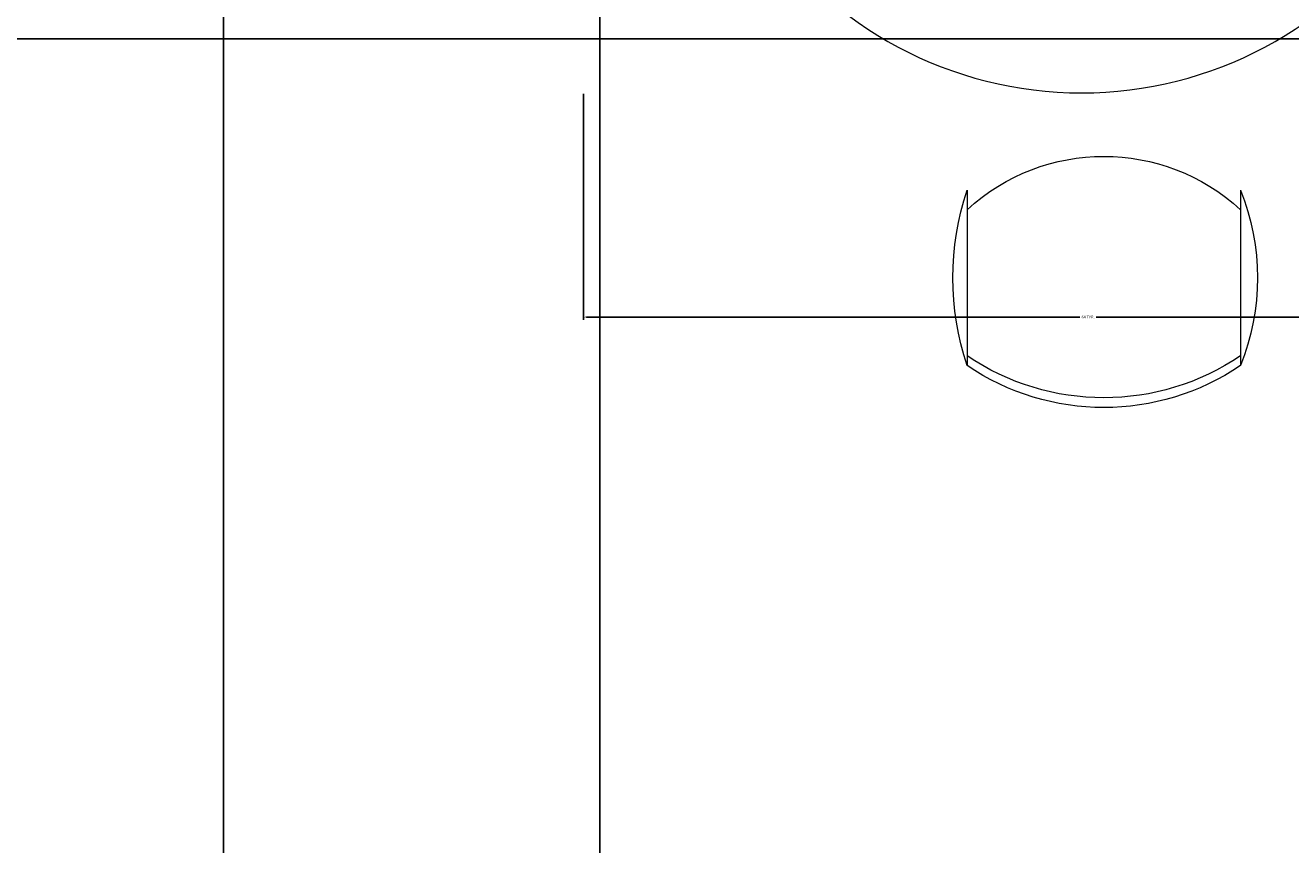
# Model space of a CAD drawing. Units: inches. Extents: x -61 to 1599, y -1316 to 257.
# Tile 92 of 204: x 240 to 321, y -219 to -166. Entities that reach past the tile are written whole.
import ezdxf

# ---------------------------------------------------------------- set-up
doc = ezdxf.new("R2010")
doc.units = ezdxf.units.IN
doc.header["$MEASUREMENT"] = 0
doc.layers.add('A-ANNO-DIMS', color=2, linetype='Continuous', lineweight=18)
doc.layers.add('FURNITURE', color=83, linetype='Continuous', lineweight=18)
doc.styles.get("Standard").update_dxf_attribs({"font": 'arial.ttf'})
doc.dimstyles.get("Standard").update_dxf_attribs({"dimtxt": 0.18, "dimasz": 0.18, "dimexe": 0.18, "dimexo": 0.0625, "dimgap": 0.09, "dimtad": 0, "dimtih": 1, "dimtoh": 1, "dimdec": 0, "dimzin": 0, "dimdsep": 46, "dimlunit": 3, "dimtxsty": 'Standard', "dimcen": 0.09, "dimadec": 0, "dimazin": 0, "dimtfac": 1, "dimtdec": 0, "dimtofl": 0, "dimtmove": 0, "dimatfit": 3, "dimfxl": 1, "dimtolj": 1, "dimtzin": 0, "dimarcsym": 0})

# ---------------------------------------------------------------- blocks, each defined once
blk = doc.blocks.new('DINING-TABLE-OVAL')
for p, q in [((20.059, 34.258), (38.124, 65.35)), ((20.686, 45.856), (30.121, 61.177)), ((27.506, 37.684), (36.941, 53.006))]:
    blk.add_line(p, q)
for centre, radius, start, end in [((28.988, 70.072), 25.358, 35.51721, 144.48279), ((85.787, 47.892), 85.786, 154.51511, 205.48489), ((-21.854, 47.892), 80.449, 332.68902, 27.31098), ((28.988, 24.89), 24.889, 213.97533, 326.02467)]:
    blk.add_arc(centre, radius, start, end)
blk = doc.blocks.new('DINING-CHAIR')
for p, q in [((0.905, 2.156), (0.905, 13.354)), ((18.348, 2.156), (18.348, 13.354))]:
    blk.add_line(p, q)
for centre, radius, start, end in [((9.626, 0.517), 15.52, 55.80984, 124.19016), ((9.626, -0.104), 15.52, 55.80984, 124.19016), ((17.781, 7.755), 17.78, 161.64548, 198.35452), ((4.514, 7.755), 14.923, 337.96463, 22.03537), ((9.626, 12.869), 12.868, 227.33204, 312.66796)]:
    blk.add_arc(centre, radius, start, end)
blk = doc.blocks.new('*D667')
at = {"layer": 'A-ANNO-DIMS', "color": 0, "lineweight": -2, "transparency": 16777216}
for p, q in [((275.852, -170.688), (275.852, -185.12)), ((340.219, -170.688), (340.219, -185.12)), ((276.032, -184.94), (307.507, -184.94)), ((340.039, -184.94), (308.564, -184.94))]:
    blk.add_line(p, q, dxfattribs=at)
at = {"layer": 'A-ANNO-DIMS', "color": 0, "transparency": 16777216}
for points in [[(276.032, -184.91), (276.032, -184.97), (275.852, -184.94)], [(340.039, -184.91), (340.039, -184.97), (340.219, -184.94)]]:
    blk.add_solid(points, dxfattribs=at)
at = {"layer": 'DEFPOINTS', "color": 0, "transparency": 16777216}
for p in [(275.852, -170.626), (340.219, -170.626), (340.219, -184.94)]:
    blk.add_point(p, dxfattribs=at)
at = {"layer": 'A-ANNO-DIMS', "color": 0, "transparency": 16777216, "insert": (308.035, -184.94), "char_height": 0.18, "attachment_point": 5}
blk.add_mtext('\\A1;64 TYP.', dxfattribs=at)
blk = doc.blocks.new('*D687')
at = {"layer": 'A-ANNO-DIMS', "color": 0, "lineweight": -2, "transparency": 16777216}
for p, q in [((289.418, 181.677), (-61.077, 181.677)), ((-60.897, 181.497), (-60.897, -528.952)), ((-60.897, -1239.765), (-60.897, -529.316)), ((319.64, -1239.945), (-61.077, -1239.945))]:
    blk.add_line(p, q, dxfattribs=at)
at = {"layer": 'A-ANNO-DIMS', "color": 0, "transparency": 16777216}
for points in [[(-60.927, 181.497), (-60.867, 181.497), (-60.897, 181.677)], [(-60.927, -1239.765), (-60.867, -1239.765), (-60.897, -1239.945)]]:
    blk.add_solid(points, dxfattribs=at)
at = {"layer": 'DEFPOINTS', "color": 0, "transparency": 16777216}
for p in [(289.481, 181.677), (-60.897, -1239.945), (319.703, -1239.945)]:
    blk.add_point(p, dxfattribs=at)
at = {"layer": 'A-ANNO-DIMS', "color": 0, "transparency": 16777216, "insert": (-60.897, -529.134), "char_height": 0.18, "attachment_point": 5}
blk.add_mtext('\\A1;1421.6', dxfattribs=at)
blk = doc.blocks.new('*D699')
at = {"layer": 'A-ANNO-DIMS', "color": 0, "lineweight": -2, "transparency": 16777216}
for p, q in [((835.64, -167.169), (-61.077, -167.169)), ((-60.897, -167.349), (-60.897, -306.726)), ((-60.897, -446.466), (-60.897, -307.09)), ((841.64, -446.646), (-61.077, -446.646))]:
    blk.add_line(p, q, dxfattribs=at)
at = {"layer": 'A-ANNO-DIMS', "color": 0, "transparency": 16777216}
for points in [[(-60.927, -167.349), (-60.867, -167.349), (-60.897, -167.169)], [(-60.927, -446.466), (-60.867, -446.466), (-60.897, -446.646)]]:
    blk.add_solid(points, dxfattribs=at)
at = {"layer": 'DEFPOINTS', "color": 0, "transparency": 16777216}
for p in [(835.703, -167.169), (-60.897, -446.646), (841.703, -446.646)]:
    blk.add_point(p, dxfattribs=at)
at = {"layer": 'A-ANNO-DIMS', "color": 0, "transparency": 16777216, "insert": (-60.897, -306.908), "char_height": 0.18, "attachment_point": 5}
blk.add_mtext('\\A1;279.5', dxfattribs=at)
blk = doc.blocks.new('*D701')
at = {"layer": 'A-ANNO-DIMS', "color": 0, "lineweight": -2, "transparency": 16777216}
for p, q in [((215.752, -616.882), (215.752, 257.457)), ((215.932, 257.277), (233.924, 257.277)), ((252.702, 257.277), (234.711, 257.277)), ((252.882, -616.882), (252.882, 257.457))]:
    blk.add_line(p, q, dxfattribs=at)
at = {"layer": 'A-ANNO-DIMS', "color": 0, "transparency": 16777216}
for points in [[(215.932, 257.307), (215.932, 257.247), (215.752, 257.277)], [(252.702, 257.307), (252.702, 257.247), (252.882, 257.277)]]:
    blk.add_solid(points, dxfattribs=at)
at = {"layer": 'DEFPOINTS', "color": 0, "transparency": 16777216}
for p in [(252.882, 257.277), (215.752, -616.945), (252.882, -616.945)]:
    blk.add_point(p, dxfattribs=at)
at = {"layer": 'A-ANNO-DIMS', "color": 0, "transparency": 16777216, "insert": (234.317, 257.277), "char_height": 0.18, "attachment_point": 5}
blk.add_mtext('\\A1;37.13', dxfattribs=at)
blk = doc.blocks.new('*D702')
at = {"layer": 'A-ANNO-DIMS', "color": 0, "lineweight": -2, "transparency": 16777216}
for p, q in [((276.882, -616.882), (276.882, 257.457)), ((277.062, 257.277), (312.209, 257.277)), ((348.14, 257.277), (312.994, 257.277)), ((348.32, -616.882), (348.32, 257.457))]:
    blk.add_line(p, q, dxfattribs=at)
at = {"layer": 'A-ANNO-DIMS', "color": 0, "transparency": 16777216}
for points in [[(277.062, 257.307), (277.062, 257.247), (276.882, 257.277)], [(348.14, 257.307), (348.14, 257.247), (348.32, 257.277)]]:
    blk.add_solid(points, dxfattribs=at)
at = {"layer": 'DEFPOINTS', "color": 0, "transparency": 16777216}
for p in [(348.32, 257.277), (276.882, -616.945), (348.32, -616.945)]:
    blk.add_point(p, dxfattribs=at)
at = {"layer": 'A-ANNO-DIMS', "color": 0, "transparency": 16777216, "insert": (312.601, 257.277), "char_height": 0.18, "attachment_point": 5}
blk.add_mtext('\\A1;71.44', dxfattribs=at)

msp = doc.modelspace()

# ---------------------------------------------------------------- block references
at = {"layer": 'FURNITURE'}
msp.add_blockref('DINING-TABLE-OVAL', (278.634, -170.626), dxfattribs=at)
at = {"layer": 'FURNITURE', "extrusion": (0, 0, -1), "zscale": -1, "rotation": 180}
msp.add_blockref('DINING-CHAIR', (-299.4166, -174.6778), dxfattribs=at)

# ---------------------------------------------------------------- dimensions: what is measured, and where the dimension line sits
at = {"layer": 'A-ANNO-DIMS'}
for base, p1, p2, picture, middle in [((252.8825, 257.2771), (215.7521, -616.9446), (252.8825, -616.9446), '*D701', (234.3173, 257.2771)), ((348.3201, 257.2771), (276.8825, -616.9446), (348.3201, -616.9446), '*D702', (312.6013, 257.2771))]:
    dim = msp.add_linear_dim(base=base, p1=p1, p2=p2, dimstyle='Standard', override={"dimdec": 2, "dimlfac": 1, "dimrnd": 0, "dimzin": 0, "dimdsep": 46, "dimlunit": 2}, dxfattribs=at)
    dim.commit()
    dim.dimension.update_dxf_attribs({"geometry": picture, "text_midpoint": middle})
for base, p1, p2, picture, middle in [((-60.8972, -1239.9446), (289.4807, 181.6771), (319.7028, -1239.9446), '*D687', (-60.8972, -529.1337)), ((-60.8972, -446.6462), (835.7028, -167.169), (841.7028, -446.6462), '*D699', (-60.8972, -306.9076))]:
    dim = msp.add_linear_dim(base=base, p1=p1, p2=p2, angle=90, dimstyle='Standard', override={"dimdec": 1, "dimlfac": 1, "dimrnd": 0, "dimzin": 0, "dimdsep": 46, "dimlunit": 2}, dxfattribs=at)
    dim.commit()
    dim.dimension.update_dxf_attribs({"geometry": picture, "text_midpoint": middle})
dim = msp.add_linear_dim(base=(340.2185, -184.9401), p1=(275.8519, -170.6256), p2=(340.2185, -170.6256), text='<> TYP.', dimstyle='Standard', override={"dimdec": 0, "dimlfac": 1, "dimrnd": 0, "dimzin": 0, "dimdsep": 46, "dimlunit": 2}, dxfattribs=at)
dim.commit()
dim.dimension.update_dxf_attribs({"geometry": '*D667', "text_midpoint": (308.0352, -184.9401)})

doc.saveas('drawing.dxf')
